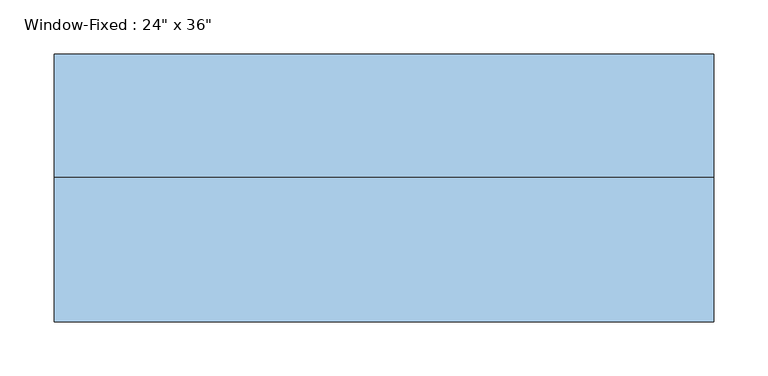
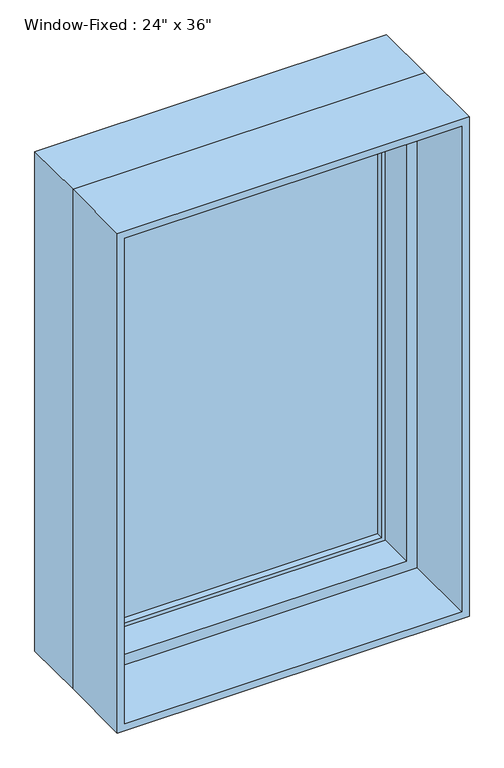
"""IFC4 building model written with IfcOpenShell, lengths in millimetres: window geometry."""

from ifc_helpers import new_model, si_unit, frame, origin, place, context, project, spatial, polyline, outline, extrude, faceted_brep, source, transform, mapped, element, save


def window_b8e47f08(model_context):
    return source(origin(), model_context, "Body", "SolidModel", [
        extrude(outline(polyline([(266.7, 114.3), (266.7, 107.95), (-266.7, 107.95), (-266.7, 114.3), (266.7, 114.3)])), frame((0.0, 0.0, 952.5), z_axis=(0.0, 0.0, 1.0), x_axis=(1.0, 0.0, 0.0)), (0.0, 0.0, 1.0), 838.2),
        extrude(outline(polyline([(-266.7, 95.25), (-266.7, 101.6), (266.7, 101.6), (266.7, 95.25), (-266.7, 95.25)])), frame((0.0, 0.0, 952.5), z_axis=(0.0, 0.0, 1.0), x_axis=(1.0, 0.0, 0.0)), (0.0, 0.0, 1.0), 838.2),
        extrude(outline(polyline([(927.1, 292.1), (1816.1, 292.1), (1816.1, -292.1), (927.1, -292.1), (927.1, 292.1)]), holes=[polyline([(952.5, -266.7), (1790.7, -266.7), (1790.7, 266.7), (952.5, 266.7), (952.5, -266.7)])]), frame((0.0, 82.55, 0.0), z_axis=(0.0, 1.0, 0.0), x_axis=(0.0, 0.0, 1.0)), (0.0, 0.0, 1.0), 44.45),
        extrude(outline(polyline([(1828.8, -304.8), (914.4, -304.8), (914.4, 304.8), (1828.8, 304.8), (1828.8, -304.8)]), holes=[polyline([(1816.1, 292.1), (927.1, 292.1), (927.1, -292.1), (1816.1, -292.1), (1816.1, 292.1)])]), frame((0.0, -114.3, 0.0), z_axis=(0.0, 1.0, 0.0), x_axis=(0.0, 0.0, 1.0)), (0.0, 0.0, 1.0), 133.35),
        faceted_brep([(304.8, 19.05, 1828.8), (304.8, 133.35, 1828.8), (-304.8, 133.35, 1828.8), (-304.8, 19.05, 1828.8), (-304.8, 133.35, 914.4), (-304.8, 19.05, 914.4), (304.8, 133.35, 914.4), (304.8, 19.05, 914.4), (273.05, 19.05, 1797.05), (273.05, 19.05, 946.15), (-273.05, 19.05, 946.15), (-273.05, 19.05, 1797.05), (-292.1, 133.35, 1816.1), (-292.1, 133.35, 927.1), (292.1, 133.35, 927.1), (292.1, 133.35, 1816.1), (273.05, 82.55, 1797.05), (-273.05, 82.55, 1797.05), (292.1, 82.55, 1816.1), (-292.1, 82.55, 1816.1), (-273.05, 82.55, 946.15), (-292.1, 82.55, 927.1), (273.05, 82.55, 946.15), (292.1, 82.55, 927.1)], [[[0, 1, 2, 3]], [[3, 2, 4, 5]], [[5, 4, 6, 7]], [[3, 5, 7, 0], [8, 9, 10, 11]], [[7, 6, 1, 0]], [[1, 6, 4, 2], [12, 13, 14, 15]], [[16, 8, 11, 17]], [[15, 18, 19, 12]], [[17, 11, 10, 20]], [[12, 19, 21, 13]], [[20, 10, 9, 22]], [[13, 21, 23, 14]], [[22, 9, 8, 16]], [[18, 23, 21, 19], [17, 20, 22, 16]], [[14, 23, 18, 15]]]),
    ])


if __name__ == "__main__":
    model = new_model("IFC4")
    model_context = context("Model", 3, world=origin())
    ifc_project = project(units=[si_unit("LENGTHUNIT", "METRE", prefix="MILLI")], contexts=[model_context])
    site = spatial("IfcSite", under=ifc_project)
    building = spatial("IfcBuilding", under=site)
    placement = place(None, origin())
    window_shape = window_b8e47f08(model_context)
    element("IfcWindow", 1, ObjectType="Window-Fixed : 24\" x 36\"", at=placement, inside=building, context=model_context, shape_type="MappedRepresentation", body=[
        mapped(window_shape, transform((0.0, 0.0, 0.0), x_axis=(1.0, 0.0, 0.0), y_axis=(0.0, 1.0, 0.0), z_axis=(0.0, 0.0, 1.0))),
    ])
    save(model, "model.ifc")

# Revit data of these elements
# Type "Window-Fixed : 24\" x 36\""
#   Type Mark = "18"
#   Fire Rating = "0.5h"
#   Assembly Code = "B2020100"
#   Analytic Construction = "Double glazing - domestic"
#   Window Inset [instance default] = 0' - 0"
#   Wall Thickness [instance default] = 0' - 6"
#   Visual Light Transmittance = 0.81
#   Thermal Resistance (R) = 1.8146 (h·ft²·°F)/BTU
#   Solar Heat Gain Coefficient = 0.76
#   Rough Width = 2' - 0 1/2"
#   Rough Height = 3' - 0 1/2"
#   Interior Wall Closure [instance default] = 0' - 2 1/4"
#   Height = 3' - 0"
#   Heat Transfer Coefficient (U) = 0.5511 BTU/(h·ft²·°F)
#   Frame Extension [instance default] = 0' - 0 1/4"
#   Exterior Wall Closure [instance default] = 0' - 1 1/4"
#   Extension Jamb [instance default] = 0' - 2 1/4"
#   Default Sill Height = 3' - 0"
#   Width = 2' - 0"
#   Muntin Visibility = yes
#   Interior Trim Visibility [instance default] = yes
#   Exterior Trim Visibility [instance default] = yes
#   Extension Jamb Visibility [instance default] = yes
#   Define Thermal Properties by = 1
#   Muntin Pattern = Muntin Pattern_2x2 : Muntin Pattern_2x2
#   Interior Trim Material = Wood - Stained
#   Interior Trim = Trim-Window-Interior-Flat : Picture Frame
#   Interior Frame Material = Wood - Stained
#   Glass Panel Material = Glass
#   Exterior Trim Material = Clad - White
#   Exterior Trim = Trim-Window-Exterior-Flat : with Sill
#   Exterior Frame Material = Clad - White
#   Wall Closure = (empty or 0)
# Element 1 (IfcWindow, "Window-Fixed : 24\" x 36\"")
#   Wall Thickness = 0' - 9"
#   Extension Jamb = 0' - 5 1/4"
#   Materials on its faces: "Wood - Stained", "Glass", "Clad - White"
# Materials
#   "Wood - Stained": class "Wood", colour RGB 173 132 96, transparency 0, Cost = 0
#   "Glass": class "Glass", colour RGB 245 245 243, transparency 1, Description = "Soda Lime Glass", Cost = 0
#   "Clad - White": class "Wood", colour RGB 245 245 243, transparency 0, Cost = 0
